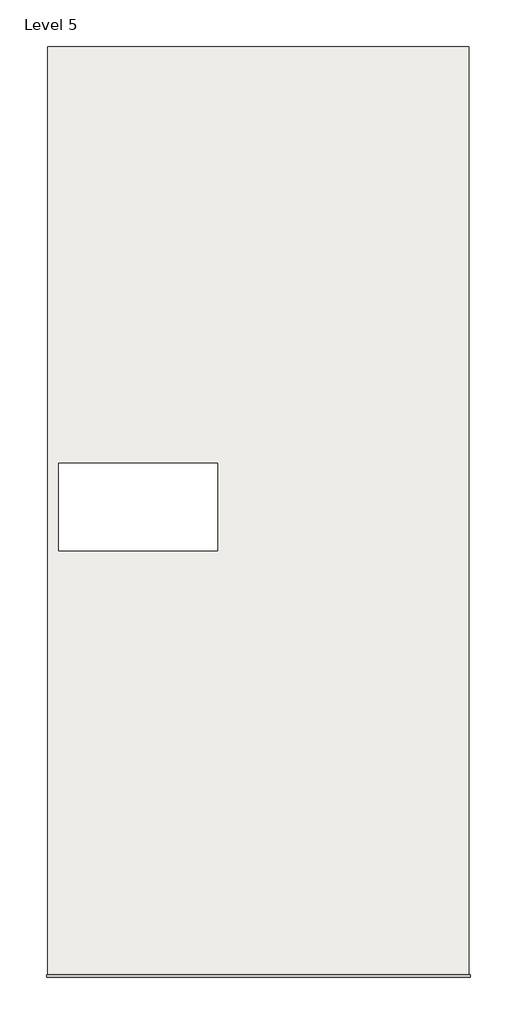
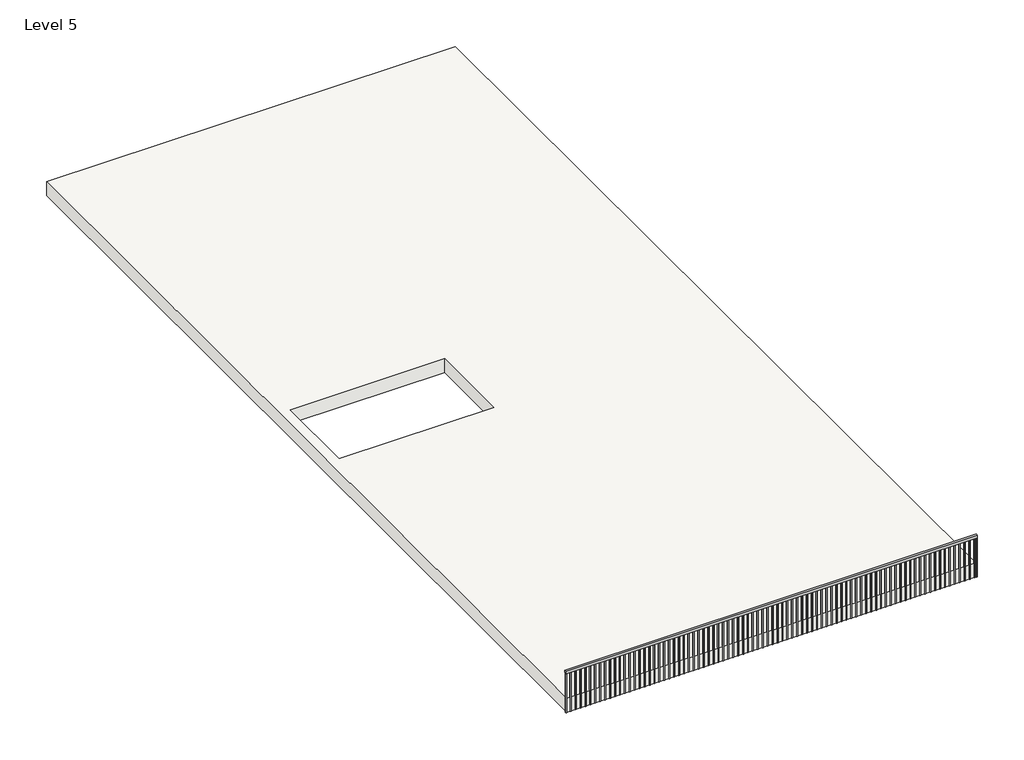
# One storey, incomplete: 1 railing, 1 roof.
"""IFC4 building model written with IfcOpenShell, lengths in millimetres."""

from ifc_helpers import new_model, si_unit, frame, origin, place, context, project, spatial, polyline, outline, extrude, element, save

model = new_model("IFC4")

# Units and contexts
model_context = context("Model", 3, world=origin())
ifc_project = project(units=[si_unit("LENGTHUNIT", "METRE", prefix="MILLI")], contexts=[model_context])

# Site, building, storey
site = spatial("IfcSite", under=ifc_project)
building = spatial("IfcBuilding", under=site)
storey = spatial("IfcBuildingStorey", under=building, Name="Level 5", Elevation=12192.0)

# Railing
placement = place(None, origin())
element("IfcRailing", 1, ObjectType="Handrail - Rectangular", at=placement, inside=storey, context=model_context, shape_type="SweptSolid", body=[
    extrude(outline(polyline([(-5185.2394105, -9094.4202879), (-5185.2394105, -9043.6202879), (3298.3605895, -9043.6202879), (3298.3605895, -9094.4202879), (-5185.2394105, -9094.4202879)])), frame((0.0, 0.0, 13055.6), z_axis=(0.0, 0.0, 1.0), x_axis=(1.0, 0.0, 0.0)), (0.0, 0.0, 1.0), 50.8),
    extrude(outline(polyline([(3238.0355895, -9078.5452879), (3238.0355895, -9059.4952879), (3257.0855895, -9059.4952879), (3257.0855895, -9078.5452879), (3238.0355895, -9078.5452879)])), frame((0.0, 0.0, 12192.0), z_axis=(0.0, 0.0, 1.0), x_axis=(1.0, 0.0, 0.0)), (0.0, 0.0, 1.0), 863.6),
    extrude(outline(polyline([(3136.4355895, -9078.5452879), (3136.4355895, -9059.4952879), (3155.4855895, -9059.4952879), (3155.4855895, -9078.5452879), (3136.4355895, -9078.5452879)])), frame((0.0, 0.0, 12192.0), z_axis=(0.0, 0.0, 1.0), x_axis=(1.0, 0.0, 0.0)), (0.0, 0.0, 1.0), 863.6),
    extrude(outline(polyline([(3034.8355895, -9078.5452879), (3034.8355895, -9059.4952879), (3053.8855895, -9059.4952879), (3053.8855895, -9078.5452879), (3034.8355895, -9078.5452879)])), frame((0.0, 0.0, 12192.0), z_axis=(0.0, 0.0, 1.0), x_axis=(1.0, 0.0, 0.0)), (0.0, 0.0, 1.0), 863.6),
    extrude(outline(polyline([(2933.2355895, -9078.5452879), (2933.2355895, -9059.4952879), (2952.2855895, -9059.4952879), (2952.2855895, -9078.5452879), (2933.2355895, -9078.5452879)])), frame((0.0, 0.0, 12192.0), z_axis=(0.0, 0.0, 1.0), x_axis=(1.0, 0.0, 0.0)), (0.0, 0.0, 1.0), 863.6),
    extrude(outline(polyline([(2831.6355895, -9078.5452879), (2831.6355895, -9059.4952879), (2850.6855895, -9059.4952879), (2850.6855895, -9078.5452879), (2831.6355895, -9078.5452879)])), frame((0.0, 0.0, 12192.0), z_axis=(0.0, 0.0, 1.0), x_axis=(1.0, 0.0, 0.0)), (0.0, 0.0, 1.0), 863.6),
    extrude(outline(polyline([(2730.0355895, -9078.5452879), (2730.0355895, -9059.4952879), (2749.0855895, -9059.4952879), (2749.0855895, -9078.5452879), (2730.0355895, -9078.5452879)])), frame((0.0, 0.0, 12192.0), z_axis=(0.0, 0.0, 1.0), x_axis=(1.0, 0.0, 0.0)), (0.0, 0.0, 1.0), 863.6),
    extrude(outline(polyline([(2628.4355895, -9078.5452879), (2628.4355895, -9059.4952879), (2647.4855895, -9059.4952879), (2647.4855895, -9078.5452879), (2628.4355895, -9078.5452879)])), frame((0.0, 0.0, 12192.0), z_axis=(0.0, 0.0, 1.0), x_axis=(1.0, 0.0, 0.0)), (0.0, 0.0, 1.0), 863.6),
    extrude(outline(polyline([(2526.8355895, -9078.5452879), (2526.8355895, -9059.4952879), (2545.8855895, -9059.4952879), (2545.8855895, -9078.5452879), (2526.8355895, -9078.5452879)])), frame((0.0, 0.0, 12192.0), z_axis=(0.0, 0.0, 1.0), x_axis=(1.0, 0.0, 0.0)), (0.0, 0.0, 1.0), 863.6),
    extrude(outline(polyline([(2425.2355895, -9078.5452879), (2425.2355895, -9059.4952879), (2444.2855895, -9059.4952879), (2444.2855895, -9078.5452879), (2425.2355895, -9078.5452879)])), frame((0.0, 0.0, 12192.0), z_axis=(0.0, 0.0, 1.0), x_axis=(1.0, 0.0, 0.0)), (0.0, 0.0, 1.0), 863.6),
    extrude(outline(polyline([(2323.6355895, -9078.5452879), (2323.6355895, -9059.4952879), (2342.6855895, -9059.4952879), (2342.6855895, -9078.5452879), (2323.6355895, -9078.5452879)])), frame((0.0, 0.0, 12192.0), z_axis=(0.0, 0.0, 1.0), x_axis=(1.0, 0.0, 0.0)), (0.0, 0.0, 1.0), 863.6),
    extrude(outline(polyline([(2222.0355895, -9078.5452879), (2222.0355895, -9059.4952879), (2241.0855895, -9059.4952879), (2241.0855895, -9078.5452879), (2222.0355895, -9078.5452879)])), frame((0.0, 0.0, 12192.0), z_axis=(0.0, 0.0, 1.0), x_axis=(1.0, 0.0, 0.0)), (0.0, 0.0, 1.0), 863.6),
    extrude(outline(polyline([(2120.4355895, -9078.5452879), (2120.4355895, -9059.4952879), (2139.4855895, -9059.4952879), (2139.4855895, -9078.5452879), (2120.4355895, -9078.5452879)])), frame((0.0, 0.0, 12192.0), z_axis=(0.0, 0.0, 1.0), x_axis=(1.0, 0.0, 0.0)), (0.0, 0.0, 1.0), 863.6),
    extrude(outline(polyline([(2018.8355895, -9078.5452879), (2018.8355895, -9059.4952879), (2037.8855895, -9059.4952879), (2037.8855895, -9078.5452879), (2018.8355895, -9078.5452879)])), frame((0.0, 0.0, 12192.0), z_axis=(0.0, 0.0, 1.0), x_axis=(1.0, 0.0, 0.0)), (0.0, 0.0, 1.0), 863.6),
    extrude(outline(polyline([(1917.2355895, -9078.5452879), (1917.2355895, -9059.4952879), (1936.2855895, -9059.4952879), (1936.2855895, -9078.5452879), (1917.2355895, -9078.5452879)])), frame((0.0, 0.0, 12192.0), z_axis=(0.0, 0.0, 1.0), x_axis=(1.0, 0.0, 0.0)), (0.0, 0.0, 1.0), 863.6),
    extrude(outline(polyline([(1815.6355895, -9078.5452879), (1815.6355895, -9059.4952879), (1834.6855895, -9059.4952879), (1834.6855895, -9078.5452879), (1815.6355895, -9078.5452879)])), frame((0.0, 0.0, 12192.0), z_axis=(0.0, 0.0, 1.0), x_axis=(1.0, 0.0, 0.0)), (0.0, 0.0, 1.0), 863.6),
    extrude(outline(polyline([(1714.0355895, -9078.5452879), (1714.0355895, -9059.4952879), (1733.0855895, -9059.4952879), (1733.0855895, -9078.5452879), (1714.0355895, -9078.5452879)])), frame((0.0, 0.0, 12192.0), z_axis=(0.0, 0.0, 1.0), x_axis=(1.0, 0.0, 0.0)), (0.0, 0.0, 1.0), 863.6),
    extrude(outline(polyline([(1612.4355895, -9078.5452879), (1612.4355895, -9059.4952879), (1631.4855895, -9059.4952879), (1631.4855895, -9078.5452879), (1612.4355895, -9078.5452879)])), frame((0.0, 0.0, 12192.0), z_axis=(0.0, 0.0, 1.0), x_axis=(1.0, 0.0, 0.0)), (0.0, 0.0, 1.0), 863.6),
    extrude(outline(polyline([(1510.8355895, -9078.5452879), (1510.8355895, -9059.4952879), (1529.8855895, -9059.4952879), (1529.8855895, -9078.5452879), (1510.8355895, -9078.5452879)])), frame((0.0, 0.0, 12192.0), z_axis=(0.0, 0.0, 1.0), x_axis=(1.0, 0.0, 0.0)), (0.0, 0.0, 1.0), 863.6),
    extrude(outline(polyline([(1409.2355895, -9078.5452879), (1409.2355895, -9059.4952879), (1428.2855895, -9059.4952879), (1428.2855895, -9078.5452879), (1409.2355895, -9078.5452879)])), frame((0.0, 0.0, 12192.0), z_axis=(0.0, 0.0, 1.0), x_axis=(1.0, 0.0, 0.0)), (0.0, 0.0, 1.0), 863.6),
    extrude(outline(polyline([(1307.6355895, -9078.5452879), (1307.6355895, -9059.4952879), (1326.6855895, -9059.4952879), (1326.6855895, -9078.5452879), (1307.6355895, -9078.5452879)])), frame((0.0, 0.0, 12192.0), z_axis=(0.0, 0.0, 1.0), x_axis=(1.0, 0.0, 0.0)), (0.0, 0.0, 1.0), 863.6),
    extrude(outline(polyline([(1206.0355895, -9078.5452879), (1206.0355895, -9059.4952879), (1225.0855895, -9059.4952879), (1225.0855895, -9078.5452879), (1206.0355895, -9078.5452879)])), frame((0.0, 0.0, 12192.0), z_axis=(0.0, 0.0, 1.0), x_axis=(1.0, 0.0, 0.0)), (0.0, 0.0, 1.0), 863.6),
    extrude(outline(polyline([(1104.4355895, -9078.5452879), (1104.4355895, -9059.4952879), (1123.4855895, -9059.4952879), (1123.4855895, -9078.5452879), (1104.4355895, -9078.5452879)])), frame((0.0, 0.0, 12192.0), z_axis=(0.0, 0.0, 1.0), x_axis=(1.0, 0.0, 0.0)), (0.0, 0.0, 1.0), 863.6),
    extrude(outline(polyline([(1002.8355895, -9078.5452879), (1002.8355895, -9059.4952879), (1021.8855895, -9059.4952879), (1021.8855895, -9078.5452879), (1002.8355895, -9078.5452879)])), frame((0.0, 0.0, 12192.0), z_axis=(0.0, 0.0, 1.0), x_axis=(1.0, 0.0, 0.0)), (0.0, 0.0, 1.0), 863.6),
    extrude(outline(polyline([(901.2355895, -9078.5452879), (901.2355895, -9059.4952879), (920.2855895, -9059.4952879), (920.2855895, -9078.5452879), (901.2355895, -9078.5452879)])), frame((0.0, 0.0, 12192.0), z_axis=(0.0, 0.0, 1.0), x_axis=(1.0, 0.0, 0.0)), (0.0, 0.0, 1.0), 863.6),
    extrude(outline(polyline([(799.6355895, -9078.5452879), (799.6355895, -9059.4952879), (818.6855895, -9059.4952879), (818.6855895, -9078.5452879), (799.6355895, -9078.5452879)])), frame((0.0, 0.0, 12192.0), z_axis=(0.0, 0.0, 1.0), x_axis=(1.0, 0.0, 0.0)), (0.0, 0.0, 1.0), 863.6),
    extrude(outline(polyline([(698.0355895, -9078.5452879), (698.0355895, -9059.4952879), (717.0855895, -9059.4952879), (717.0855895, -9078.5452879), (698.0355895, -9078.5452879)])), frame((0.0, 0.0, 12192.0), z_axis=(0.0, 0.0, 1.0), x_axis=(1.0, 0.0, 0.0)), (0.0, 0.0, 1.0), 863.6),
    extrude(outline(polyline([(596.4355895, -9078.5452879), (596.4355895, -9059.4952879), (615.4855895, -9059.4952879), (615.4855895, -9078.5452879), (596.4355895, -9078.5452879)])), frame((0.0, 0.0, 12192.0), z_axis=(0.0, 0.0, 1.0), x_axis=(1.0, 0.0, 0.0)), (0.0, 0.0, 1.0), 863.6),
    extrude(outline(polyline([(494.8355895, -9078.5452879), (494.8355895, -9059.4952879), (513.8855895, -9059.4952879), (513.8855895, -9078.5452879), (494.8355895, -9078.5452879)])), frame((0.0, 0.0, 12192.0), z_axis=(0.0, 0.0, 1.0), x_axis=(1.0, 0.0, 0.0)), (0.0, 0.0, 1.0), 863.6),
    extrude(outline(polyline([(393.2355895, -9078.5452879), (393.2355895, -9059.4952879), (412.2855895, -9059.4952879), (412.2855895, -9078.5452879), (393.2355895, -9078.5452879)])), frame((0.0, 0.0, 12192.0), z_axis=(0.0, 0.0, 1.0), x_axis=(1.0, 0.0, 0.0)), (0.0, 0.0, 1.0), 863.6),
    extrude(outline(polyline([(291.6355895, -9078.5452879), (291.6355895, -9059.4952879), (310.6855895, -9059.4952879), (310.6855895, -9078.5452879), (291.6355895, -9078.5452879)])), frame((0.0, 0.0, 12192.0), z_axis=(0.0, 0.0, 1.0), x_axis=(1.0, 0.0, 0.0)), (0.0, 0.0, 1.0), 863.6),
    extrude(outline(polyline([(190.0355895, -9078.5452879), (190.0355895, -9059.4952879), (209.0855895, -9059.4952879), (209.0855895, -9078.5452879), (190.0355895, -9078.5452879)])), frame((0.0, 0.0, 12192.0), z_axis=(0.0, 0.0, 1.0), x_axis=(1.0, 0.0, 0.0)), (0.0, 0.0, 1.0), 863.6),
    extrude(outline(polyline([(88.4355895, -9078.5452879), (88.4355895, -9059.4952879), (107.4855895, -9059.4952879), (107.4855895, -9078.5452879), (88.4355895, -9078.5452879)])), frame((0.0, 0.0, 12192.0), z_axis=(0.0, 0.0, 1.0), x_axis=(1.0, 0.0, 0.0)), (0.0, 0.0, 1.0), 863.6),
    extrude(outline(polyline([(-13.1644105, -9078.5452879), (-13.1644105, -9059.4952879), (5.8855895, -9059.4952879), (5.8855895, -9078.5452879), (-13.1644105, -9078.5452879)])), frame((0.0, 0.0, 12192.0), z_axis=(0.0, 0.0, 1.0), x_axis=(1.0, 0.0, 0.0)), (0.0, 0.0, 1.0), 863.6),
    extrude(outline(polyline([(-114.7644105, -9078.5452879), (-114.7644105, -9059.4952879), (-95.7144105, -9059.4952879), (-95.7144105, -9078.5452879), (-114.7644105, -9078.5452879)])), frame((0.0, 0.0, 12192.0), z_axis=(0.0, 0.0, 1.0), x_axis=(1.0, 0.0, 0.0)), (0.0, 0.0, 1.0), 863.6),
    extrude(outline(polyline([(-216.3644105, -9078.5452879), (-216.3644105, -9059.4952879), (-197.3144105, -9059.4952879), (-197.3144105, -9078.5452879), (-216.3644105, -9078.5452879)])), frame((0.0, 0.0, 12192.0), z_axis=(0.0, 0.0, 1.0), x_axis=(1.0, 0.0, 0.0)), (0.0, 0.0, 1.0), 863.6),
    extrude(outline(polyline([(-317.9644105, -9078.5452879), (-317.9644105, -9059.4952879), (-298.9144105, -9059.4952879), (-298.9144105, -9078.5452879), (-317.9644105, -9078.5452879)])), frame((0.0, 0.0, 12192.0), z_axis=(0.0, 0.0, 1.0), x_axis=(1.0, 0.0, 0.0)), (0.0, 0.0, 1.0), 863.6),
    extrude(outline(polyline([(-419.5644105, -9078.5452879), (-419.5644105, -9059.4952879), (-400.5144105, -9059.4952879), (-400.5144105, -9078.5452879), (-419.5644105, -9078.5452879)])), frame((0.0, 0.0, 12192.0), z_axis=(0.0, 0.0, 1.0), x_axis=(1.0, 0.0, 0.0)), (0.0, 0.0, 1.0), 863.6),
    extrude(outline(polyline([(-521.1644105, -9078.5452879), (-521.1644105, -9059.4952879), (-502.1144105, -9059.4952879), (-502.1144105, -9078.5452879), (-521.1644105, -9078.5452879)])), frame((0.0, 0.0, 12192.0), z_axis=(0.0, 0.0, 1.0), x_axis=(1.0, 0.0, 0.0)), (0.0, 0.0, 1.0), 863.6),
    extrude(outline(polyline([(-622.7644105, -9078.5452879), (-622.7644105, -9059.4952879), (-603.7144105, -9059.4952879), (-603.7144105, -9078.5452879), (-622.7644105, -9078.5452879)])), frame((0.0, 0.0, 12192.0), z_axis=(0.0, 0.0, 1.0), x_axis=(1.0, 0.0, 0.0)), (0.0, 0.0, 1.0), 863.6),
    extrude(outline(polyline([(-724.3644105, -9078.5452879), (-724.3644105, -9059.4952879), (-705.3144105, -9059.4952879), (-705.3144105, -9078.5452879), (-724.3644105, -9078.5452879)])), frame((0.0, 0.0, 12192.0), z_axis=(0.0, 0.0, 1.0), x_axis=(1.0, 0.0, 0.0)), (0.0, 0.0, 1.0), 863.6),
    extrude(outline(polyline([(-825.9644105, -9078.5452879), (-825.9644105, -9059.4952879), (-806.9144105, -9059.4952879), (-806.9144105, -9078.5452879), (-825.9644105, -9078.5452879)])), frame((0.0, 0.0, 12192.0), z_axis=(0.0, 0.0, 1.0), x_axis=(1.0, 0.0, 0.0)), (0.0, 0.0, 1.0), 863.6),
    extrude(outline(polyline([(-927.5644105, -9078.5452879), (-927.5644105, -9059.4952879), (-908.5144105, -9059.4952879), (-908.5144105, -9078.5452879), (-927.5644105, -9078.5452879)])), frame((0.0, 0.0, 12192.0), z_axis=(0.0, 0.0, 1.0), x_axis=(1.0, 0.0, 0.0)), (0.0, 0.0, 1.0), 863.6),
    extrude(outline(polyline([(-1029.1644105, -9078.5452879), (-1029.1644105, -9059.4952879), (-1010.1144105, -9059.4952879), (-1010.1144105, -9078.5452879), (-1029.1644105, -9078.5452879)])), frame((0.0, 0.0, 12192.0), z_axis=(0.0, 0.0, 1.0), x_axis=(1.0, 0.0, 0.0)), (0.0, 0.0, 1.0), 863.6),
    extrude(outline(polyline([(-1130.7644105, -9078.5452879), (-1130.7644105, -9059.4952879), (-1111.7144105, -9059.4952879), (-1111.7144105, -9078.5452879), (-1130.7644105, -9078.5452879)])), frame((0.0, 0.0, 12192.0), z_axis=(0.0, 0.0, 1.0), x_axis=(1.0, 0.0, 0.0)), (0.0, 0.0, 1.0), 863.6),
    extrude(outline(polyline([(-1232.3644105, -9078.5452879), (-1232.3644105, -9059.4952879), (-1213.3144105, -9059.4952879), (-1213.3144105, -9078.5452879), (-1232.3644105, -9078.5452879)])), frame((0.0, 0.0, 12192.0), z_axis=(0.0, 0.0, 1.0), x_axis=(1.0, 0.0, 0.0)), (0.0, 0.0, 1.0), 863.6),
    extrude(outline(polyline([(-1333.9644105, -9078.5452879), (-1333.9644105, -9059.4952879), (-1314.9144105, -9059.4952879), (-1314.9144105, -9078.5452879), (-1333.9644105, -9078.5452879)])), frame((0.0, 0.0, 12192.0), z_axis=(0.0, 0.0, 1.0), x_axis=(1.0, 0.0, 0.0)), (0.0, 0.0, 1.0), 863.6),
    extrude(outline(polyline([(-1435.5644105, -9078.5452879), (-1435.5644105, -9059.4952879), (-1416.5144105, -9059.4952879), (-1416.5144105, -9078.5452879), (-1435.5644105, -9078.5452879)])), frame((0.0, 0.0, 12192.0), z_axis=(0.0, 0.0, 1.0), x_axis=(1.0, 0.0, 0.0)), (0.0, 0.0, 1.0), 863.6),
    extrude(outline(polyline([(-1537.1644105, -9078.5452879), (-1537.1644105, -9059.4952879), (-1518.1144105, -9059.4952879), (-1518.1144105, -9078.5452879), (-1537.1644105, -9078.5452879)])), frame((0.0, 0.0, 12192.0), z_axis=(0.0, 0.0, 1.0), x_axis=(1.0, 0.0, 0.0)), (0.0, 0.0, 1.0), 863.6),
    extrude(outline(polyline([(-1638.7644105, -9078.5452879), (-1638.7644105, -9059.4952879), (-1619.7144105, -9059.4952879), (-1619.7144105, -9078.5452879), (-1638.7644105, -9078.5452879)])), frame((0.0, 0.0, 12192.0), z_axis=(0.0, 0.0, 1.0), x_axis=(1.0, 0.0, 0.0)), (0.0, 0.0, 1.0), 863.6),
    extrude(outline(polyline([(-1740.3644105, -9078.5452879), (-1740.3644105, -9059.4952879), (-1721.3144105, -9059.4952879), (-1721.3144105, -9078.5452879), (-1740.3644105, -9078.5452879)])), frame((0.0, 0.0, 12192.0), z_axis=(0.0, 0.0, 1.0), x_axis=(1.0, 0.0, 0.0)), (0.0, 0.0, 1.0), 863.6),
    extrude(outline(polyline([(-1841.9644105, -9078.5452879), (-1841.9644105, -9059.4952879), (-1822.9144105, -9059.4952879), (-1822.9144105, -9078.5452879), (-1841.9644105, -9078.5452879)])), frame((0.0, 0.0, 12192.0), z_axis=(0.0, 0.0, 1.0), x_axis=(1.0, 0.0, 0.0)), (0.0, 0.0, 1.0), 863.6),
    extrude(outline(polyline([(-1943.5644105, -9078.5452879), (-1943.5644105, -9059.4952879), (-1924.5144105, -9059.4952879), (-1924.5144105, -9078.5452879), (-1943.5644105, -9078.5452879)])), frame((0.0, 0.0, 12192.0), z_axis=(0.0, 0.0, 1.0), x_axis=(1.0, 0.0, 0.0)), (0.0, 0.0, 1.0), 863.6),
    extrude(outline(polyline([(-2045.1644105, -9078.5452879), (-2045.1644105, -9059.4952879), (-2026.1144105, -9059.4952879), (-2026.1144105, -9078.5452879), (-2045.1644105, -9078.5452879)])), frame((0.0, 0.0, 12192.0), z_axis=(0.0, 0.0, 1.0), x_axis=(1.0, 0.0, 0.0)), (0.0, 0.0, 1.0), 863.6),
    extrude(outline(polyline([(-2146.7644105, -9078.5452879), (-2146.7644105, -9059.4952879), (-2127.7144105, -9059.4952879), (-2127.7144105, -9078.5452879), (-2146.7644105, -9078.5452879)])), frame((0.0, 0.0, 12192.0), z_axis=(0.0, 0.0, 1.0), x_axis=(1.0, 0.0, 0.0)), (0.0, 0.0, 1.0), 863.6),
    extrude(outline(polyline([(-2248.3644105, -9078.5452879), (-2248.3644105, -9059.4952879), (-2229.3144105, -9059.4952879), (-2229.3144105, -9078.5452879), (-2248.3644105, -9078.5452879)])), frame((0.0, 0.0, 12192.0), z_axis=(0.0, 0.0, 1.0), x_axis=(1.0, 0.0, 0.0)), (0.0, 0.0, 1.0), 863.6),
    extrude(outline(polyline([(-2349.9644105, -9078.5452879), (-2349.9644105, -9059.4952879), (-2330.9144105, -9059.4952879), (-2330.9144105, -9078.5452879), (-2349.9644105, -9078.5452879)])), frame((0.0, 0.0, 12192.0), z_axis=(0.0, 0.0, 1.0), x_axis=(1.0, 0.0, 0.0)), (0.0, 0.0, 1.0), 863.6),
    extrude(outline(polyline([(-2451.5644105, -9078.5452879), (-2451.5644105, -9059.4952879), (-2432.5144105, -9059.4952879), (-2432.5144105, -9078.5452879), (-2451.5644105, -9078.5452879)])), frame((0.0, 0.0, 12192.0), z_axis=(0.0, 0.0, 1.0), x_axis=(1.0, 0.0, 0.0)), (0.0, 0.0, 1.0), 863.6),
    extrude(outline(polyline([(-2553.1644105, -9078.5452879), (-2553.1644105, -9059.4952879), (-2534.1144105, -9059.4952879), (-2534.1144105, -9078.5452879), (-2553.1644105, -9078.5452879)])), frame((0.0, 0.0, 12192.0), z_axis=(0.0, 0.0, 1.0), x_axis=(1.0, 0.0, 0.0)), (0.0, 0.0, 1.0), 863.6),
    extrude(outline(polyline([(-2654.7644105, -9078.5452879), (-2654.7644105, -9059.4952879), (-2635.7144105, -9059.4952879), (-2635.7144105, -9078.5452879), (-2654.7644105, -9078.5452879)])), frame((0.0, 0.0, 12192.0), z_axis=(0.0, 0.0, 1.0), x_axis=(1.0, 0.0, 0.0)), (0.0, 0.0, 1.0), 863.6),
    extrude(outline(polyline([(-2756.3644105, -9078.5452879), (-2756.3644105, -9059.4952879), (-2737.3144105, -9059.4952879), (-2737.3144105, -9078.5452879), (-2756.3644105, -9078.5452879)])), frame((0.0, 0.0, 12192.0), z_axis=(0.0, 0.0, 1.0), x_axis=(1.0, 0.0, 0.0)), (0.0, 0.0, 1.0), 863.6),
    extrude(outline(polyline([(-2857.9644105, -9078.5452879), (-2857.9644105, -9059.4952879), (-2838.9144105, -9059.4952879), (-2838.9144105, -9078.5452879), (-2857.9644105, -9078.5452879)])), frame((0.0, 0.0, 12192.0), z_axis=(0.0, 0.0, 1.0), x_axis=(1.0, 0.0, 0.0)), (0.0, 0.0, 1.0), 863.6),
    extrude(outline(polyline([(-2959.5644105, -9078.5452879), (-2959.5644105, -9059.4952879), (-2940.5144105, -9059.4952879), (-2940.5144105, -9078.5452879), (-2959.5644105, -9078.5452879)])), frame((0.0, 0.0, 12192.0), z_axis=(0.0, 0.0, 1.0), x_axis=(1.0, 0.0, 0.0)), (0.0, 0.0, 1.0), 863.6),
    extrude(outline(polyline([(-3061.1644105, -9078.5452879), (-3061.1644105, -9059.4952879), (-3042.1144105, -9059.4952879), (-3042.1144105, -9078.5452879), (-3061.1644105, -9078.5452879)])), frame((0.0, 0.0, 12192.0), z_axis=(0.0, 0.0, 1.0), x_axis=(1.0, 0.0, 0.0)), (0.0, 0.0, 1.0), 863.6),
    extrude(outline(polyline([(-3162.7644105, -9078.5452879), (-3162.7644105, -9059.4952879), (-3143.7144105, -9059.4952879), (-3143.7144105, -9078.5452879), (-3162.7644105, -9078.5452879)])), frame((0.0, 0.0, 12192.0), z_axis=(0.0, 0.0, 1.0), x_axis=(1.0, 0.0, 0.0)), (0.0, 0.0, 1.0), 863.6),
    extrude(outline(polyline([(-3264.3644105, -9078.5452879), (-3264.3644105, -9059.4952879), (-3245.3144105, -9059.4952879), (-3245.3144105, -9078.5452879), (-3264.3644105, -9078.5452879)])), frame((0.0, 0.0, 12192.0), z_axis=(0.0, 0.0, 1.0), x_axis=(1.0, 0.0, 0.0)), (0.0, 0.0, 1.0), 863.6),
    extrude(outline(polyline([(-3365.9644105, -9078.5452879), (-3365.9644105, -9059.4952879), (-3346.9144105, -9059.4952879), (-3346.9144105, -9078.5452879), (-3365.9644105, -9078.5452879)])), frame((0.0, 0.0, 12192.0), z_axis=(0.0, 0.0, 1.0), x_axis=(1.0, 0.0, 0.0)), (0.0, 0.0, 1.0), 863.6),
    extrude(outline(polyline([(-3467.5644105, -9078.5452879), (-3467.5644105, -9059.4952879), (-3448.5144105, -9059.4952879), (-3448.5144105, -9078.5452879), (-3467.5644105, -9078.5452879)])), frame((0.0, 0.0, 12192.0), z_axis=(0.0, 0.0, 1.0), x_axis=(1.0, 0.0, 0.0)), (0.0, 0.0, 1.0), 863.6),
    extrude(outline(polyline([(-3569.1644105, -9078.5452879), (-3569.1644105, -9059.4952879), (-3550.1144105, -9059.4952879), (-3550.1144105, -9078.5452879), (-3569.1644105, -9078.5452879)])), frame((0.0, 0.0, 12192.0), z_axis=(0.0, 0.0, 1.0), x_axis=(1.0, 0.0, 0.0)), (0.0, 0.0, 1.0), 863.6),
    extrude(outline(polyline([(-3670.7644105, -9078.5452879), (-3670.7644105, -9059.4952879), (-3651.7144105, -9059.4952879), (-3651.7144105, -9078.5452879), (-3670.7644105, -9078.5452879)])), frame((0.0, 0.0, 12192.0), z_axis=(0.0, 0.0, 1.0), x_axis=(1.0, 0.0, 0.0)), (0.0, 0.0, 1.0), 863.6),
    extrude(outline(polyline([(-3772.3644105, -9078.5452879), (-3772.3644105, -9059.4952879), (-3753.3144105, -9059.4952879), (-3753.3144105, -9078.5452879), (-3772.3644105, -9078.5452879)])), frame((0.0, 0.0, 12192.0), z_axis=(0.0, 0.0, 1.0), x_axis=(1.0, 0.0, 0.0)), (0.0, 0.0, 1.0), 863.6),
    extrude(outline(polyline([(-3873.9644105, -9078.5452879), (-3873.9644105, -9059.4952879), (-3854.9144105, -9059.4952879), (-3854.9144105, -9078.5452879), (-3873.9644105, -9078.5452879)])), frame((0.0, 0.0, 12192.0), z_axis=(0.0, 0.0, 1.0), x_axis=(1.0, 0.0, 0.0)), (0.0, 0.0, 1.0), 863.6),
    extrude(outline(polyline([(-3975.5644105, -9078.5452879), (-3975.5644105, -9059.4952879), (-3956.5144105, -9059.4952879), (-3956.5144105, -9078.5452879), (-3975.5644105, -9078.5452879)])), frame((0.0, 0.0, 12192.0), z_axis=(0.0, 0.0, 1.0), x_axis=(1.0, 0.0, 0.0)), (0.0, 0.0, 1.0), 863.6),
    extrude(outline(polyline([(-4077.1644105, -9078.5452879), (-4077.1644105, -9059.4952879), (-4058.1144105, -9059.4952879), (-4058.1144105, -9078.5452879), (-4077.1644105, -9078.5452879)])), frame((0.0, 0.0, 12192.0), z_axis=(0.0, 0.0, 1.0), x_axis=(1.0, 0.0, 0.0)), (0.0, 0.0, 1.0), 863.6),
    extrude(outline(polyline([(-4178.7644105, -9078.5452879), (-4178.7644105, -9059.4952879), (-4159.7144105, -9059.4952879), (-4159.7144105, -9078.5452879), (-4178.7644105, -9078.5452879)])), frame((0.0, 0.0, 12192.0), z_axis=(0.0, 0.0, 1.0), x_axis=(1.0, 0.0, 0.0)), (0.0, 0.0, 1.0), 863.6),
    extrude(outline(polyline([(-4280.3644105, -9078.5452879), (-4280.3644105, -9059.4952879), (-4261.3144105, -9059.4952879), (-4261.3144105, -9078.5452879), (-4280.3644105, -9078.5452879)])), frame((0.0, 0.0, 12192.0), z_axis=(0.0, 0.0, 1.0), x_axis=(1.0, 0.0, 0.0)), (0.0, 0.0, 1.0), 863.6),
    extrude(outline(polyline([(-4381.9644105, -9078.5452879), (-4381.9644105, -9059.4952879), (-4362.9144105, -9059.4952879), (-4362.9144105, -9078.5452879), (-4381.9644105, -9078.5452879)])), frame((0.0, 0.0, 12192.0), z_axis=(0.0, 0.0, 1.0), x_axis=(1.0, 0.0, 0.0)), (0.0, 0.0, 1.0), 863.6),
    extrude(outline(polyline([(-4483.5644105, -9078.5452879), (-4483.5644105, -9059.4952879), (-4464.5144105, -9059.4952879), (-4464.5144105, -9078.5452879), (-4483.5644105, -9078.5452879)])), frame((0.0, 0.0, 12192.0), z_axis=(0.0, 0.0, 1.0), x_axis=(1.0, 0.0, 0.0)), (0.0, 0.0, 1.0), 863.6),
    extrude(outline(polyline([(-4585.1644105, -9078.5452879), (-4585.1644105, -9059.4952879), (-4566.1144105, -9059.4952879), (-4566.1144105, -9078.5452879), (-4585.1644105, -9078.5452879)])), frame((0.0, 0.0, 12192.0), z_axis=(0.0, 0.0, 1.0), x_axis=(1.0, 0.0, 0.0)), (0.0, 0.0, 1.0), 863.6),
    extrude(outline(polyline([(-4686.7644105, -9078.5452879), (-4686.7644105, -9059.4952879), (-4667.7144105, -9059.4952879), (-4667.7144105, -9078.5452879), (-4686.7644105, -9078.5452879)])), frame((0.0, 0.0, 12192.0), z_axis=(0.0, 0.0, 1.0), x_axis=(1.0, 0.0, 0.0)), (0.0, 0.0, 1.0), 863.6),
    extrude(outline(polyline([(-4788.3644105, -9078.5452879), (-4788.3644105, -9059.4952879), (-4769.3144105, -9059.4952879), (-4769.3144105, -9078.5452879), (-4788.3644105, -9078.5452879)])), frame((0.0, 0.0, 12192.0), z_axis=(0.0, 0.0, 1.0), x_axis=(1.0, 0.0, 0.0)), (0.0, 0.0, 1.0), 863.6),
    extrude(outline(polyline([(-4889.9644105, -9078.5452879), (-4889.9644105, -9059.4952879), (-4870.9144105, -9059.4952879), (-4870.9144105, -9078.5452879), (-4889.9644105, -9078.5452879)])), frame((0.0, 0.0, 12192.0), z_axis=(0.0, 0.0, 1.0), x_axis=(1.0, 0.0, 0.0)), (0.0, 0.0, 1.0), 863.6),
    extrude(outline(polyline([(-4991.5644105, -9078.5452879), (-4991.5644105, -9059.4952879), (-4972.5144105, -9059.4952879), (-4972.5144105, -9078.5452879), (-4991.5644105, -9078.5452879)])), frame((0.0, 0.0, 12192.0), z_axis=(0.0, 0.0, 1.0), x_axis=(1.0, 0.0, 0.0)), (0.0, 0.0, 1.0), 863.6),
    extrude(outline(polyline([(-5093.1644105, -9078.5452879), (-5093.1644105, -9059.4952879), (-5074.1144105, -9059.4952879), (-5074.1144105, -9078.5452879), (-5093.1644105, -9078.5452879)])), frame((0.0, 0.0, 12192.0), z_axis=(0.0, 0.0, 1.0), x_axis=(1.0, 0.0, 0.0)), (0.0, 0.0, 1.0), 863.6),
    extrude(outline(polyline([(3279.3105895, -9078.5452879), (3279.3105895, -9059.4952879), (3298.3605895, -9059.4952879), (3298.3605895, -9078.5452879), (3279.3105895, -9078.5452879)])), frame((0.0, 0.0, 12192.0), z_axis=(0.0, 0.0, 1.0), x_axis=(1.0, 0.0, 0.0)), (0.0, 0.0, 1.0), 863.6),
    extrude(outline(polyline([(-5185.2394105, -9078.5452879), (-5185.2394105, -9059.4952879), (-5166.1894105, -9059.4952879), (-5166.1894105, -9078.5452879), (-5185.2394105, -9078.5452879)])), frame((0.0, 0.0, 12192.0), z_axis=(0.0, 0.0, 1.0), x_axis=(1.0, 0.0, 0.0)), (0.0, 0.0, 1.0), 863.6),
])

# Roof
element("IfcRoof", 2, ObjectType="Generic - 12\"", at=placement, inside=storey, context=model_context, shape_type="SweptSolid", body=[
    extrude(outline(polyline([(3272.9605895, 9523.7797121), (3272.9605895, -9069.0202879), (-5159.8394105, -9069.0202879), (-5159.8394105, 9523.7797121), (3272.9605895, 9523.7797121)]), holes=[polyline([(-1756.1922756, 1192.5797121), (-4943.9394105, 1192.5797121), (-4943.9394105, -560.0202879), (-1756.1922756, -560.0202879), (-1756.1922756, 1192.5797121)])]), frame((0.0, 0.0, 12192.0), z_axis=(0.0, 0.0, 1.0), x_axis=(1.0, 0.0, 0.0)), (0.0, 0.0, 1.0), 304.8),
])

save(model, "model.ifc")

# Revit data of these elements
# Type "Handrail - Rectangular"
#   Assembly Code = "C2010400"
#   built-in parameter 1008612 = 0.0416667 (stored number, unit not read)
#   built-in parameter 1008611 = 0.0416667 (stored number, unit not read)
#   built-in parameter 1008609 = 0.333333 (stored number, unit not read)
#   built-in parameter 1008604 = 0.166667 (stored number, unit not read)
#   built-in parameter 1008603 = 0.166667 (stored number, unit not read)
#   Railing Height = 914.4 mm
#   built-in parameter 1008630 = 2
#   built-in parameter 1008610 = 2
#   built-in parameter 1008618 = Baluster - Square : 3/4"
# Type "Generic - 12\""
#   Assembly Code = "B1020"
#   Layers, outside or top first: 304.8 mm no material (function 1)
# Element 1 (IfcRailing, "Handrail - Rectangular")
#   Phase Created = New Construction
# Element 2 (IfcRoof, "Generic - 12\"")
#   built-in parameter 1001705 = 41 (stored number, unit not read)
#   built-in parameter 1001710 = 33615
#   Phase Created = New Construction
#   Materials on its faces: "Default Roof"
# Materials
#   "Default Roof": colour RGB 88 101 114, transparency 0, Cost = 0
